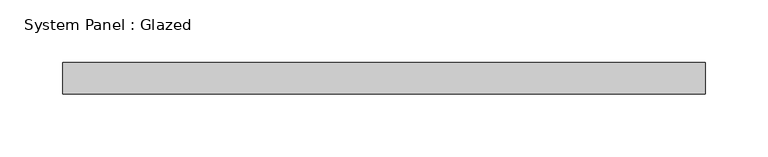
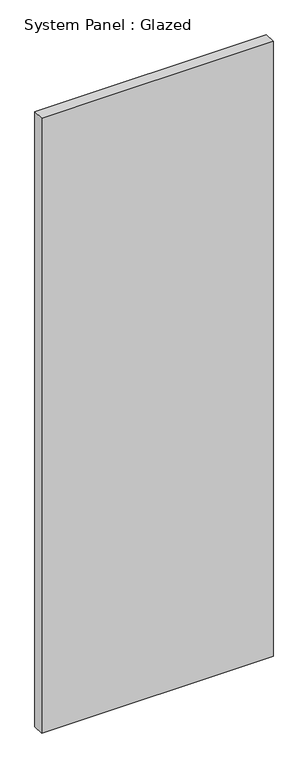
"""IFC4 building model written with IfcOpenShell, lengths in millimetres: plate geometry, System Panel : Glazed."""

from ifc_helpers import new_model, si_unit, origin, origin_with_axes, place, context, project, spatial, polyline, outline, extrude, source, transform, mapped, element, save


def system_panel_glazed_2aec2d59(model_context):
    return source(origin(), model_context, "Body", "SweptSolid", [
        extrude(outline(polyline([(257.175, 19.05), (-257.175, 19.05), (-257.175, 44.45), (257.175, 44.45), (257.175, 19.05)])), origin_with_axes(), (0.0, 0.0, 1.0), 1444.3949481),
    ])


if __name__ == "__main__":
    model = new_model("IFC4")
    model_context = context("Model", 3, world=origin())
    ifc_project = project(units=[si_unit("LENGTHUNIT", "METRE", prefix="MILLI")], contexts=[model_context])
    site = spatial("IfcSite", under=ifc_project)
    building = spatial("IfcBuilding", under=site)
    placement = place(None, origin())
    system_panel_glazed_shape = system_panel_glazed_2aec2d59(model_context)
    element("IfcPlate", 1, ObjectType="System Panel : Glazed", at=placement, inside=building, context=model_context, shape_type="MappedRepresentation", body=[
        mapped(system_panel_glazed_shape, transform((0.0, 0.0, 0.0), x_axis=(1.0, 0.0, 0.0), y_axis=(0.0, 1.0, 0.0), z_axis=(0.0, 0.0, 1.0))),
    ])
    save(model, "model.ifc")

# Revit data of these elements
# Type "System Panel : Glazed"
#   Construction Type Id = "GSP4R"
#   Analytic Construction = "1/8 in Pilkington single glazing"
#   Visual Light Transmittance = 0.9
#   Solar Heat Gain Coefficient = 0.86
#   Heat Transfer Coefficient (U) = 1.18115 BTU/(h·ft²·°F)
#   Define Thermal Properties by = 1
# Element 1 (IfcPlate, "System Panel : Glazed")
#   Materials on its faces: "Glass"
# Materials
#   "Glass": class "Glass", colour RGB 0 128 192, transparency 0.75, Description = "Soda Lime Glass", Cost = 0
